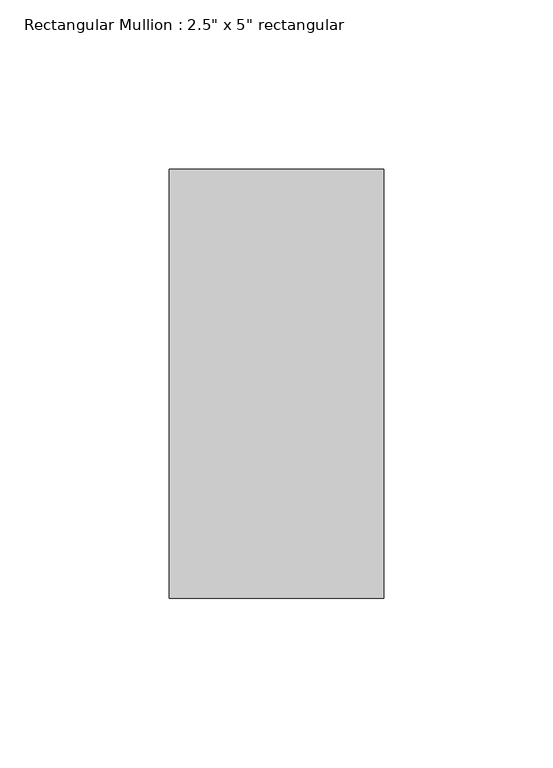
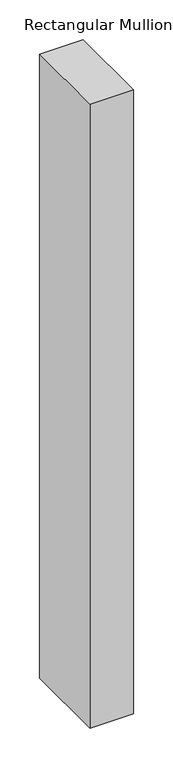
"""IFC4 building model written with IfcOpenShell, lengths in millimetres: member geometry."""

from ifc_helpers import new_model, si_unit, frame, origin, place, context, project, spatial, polyline, outline, extrude, source, transform, mapped, element, save


def member_58cc8d1f(model_context):
    return source(origin(), model_context, "Body", "SweptSolid", [
        extrude(outline(polyline([(31.75, 63.5), (31.75, -63.5), (-31.75, -63.5), (-31.75, 63.5), (31.75, 63.5)])), frame((0.0, 0.0, -960.8037122), z_axis=(0.0, 0.0, 1.0), x_axis=(1.0, 0.0, 0.0)), (0.0, 0.0, 1.0), 960.8037122),
    ])


if __name__ == "__main__":
    model = new_model("IFC4")
    model_context = context("Model", 3, world=origin())
    ifc_project = project(units=[si_unit("LENGTHUNIT", "METRE", prefix="MILLI")], contexts=[model_context])
    site = spatial("IfcSite", under=ifc_project)
    building = spatial("IfcBuilding", under=site)
    placement = place(None, origin())
    member_shape = member_58cc8d1f(model_context)
    element("IfcMember", 1, ObjectType="Rectangular Mullion : 2.5\" x 5\" rectangular", at=placement, inside=building, context=model_context, shape_type="MappedRepresentation", body=[
        mapped(member_shape, transform((0.0, 0.0, 0.0), x_axis=(1.0, 0.0, 0.0), y_axis=(0.0, 1.0, 0.0), z_axis=(0.0, 0.0, 1.0))),
    ])
    save(model, "model.ifc")

# Revit data of these elements
# Type "Rectangular Mullion : 2.5\" x 5\" rectangular"
#   built-in parameter 1007304 = 0.416667 (stored number, unit not read)
#   built-in parameter 1007301 = 0.104167 (stored number, unit not read)
#   built-in parameter 1007300 = 0.104167 (stored number, unit not read)
# Element 1 (IfcMember, "Rectangular Mullion : 2.5\" x 5\" rectangular")
#   Materials on its faces: "Aluminum"
# Materials
#   "Aluminum": class "Metal", colour RGB 247 247 247, transparency 0, Description = "Aluminum 6061", Cost = 0
